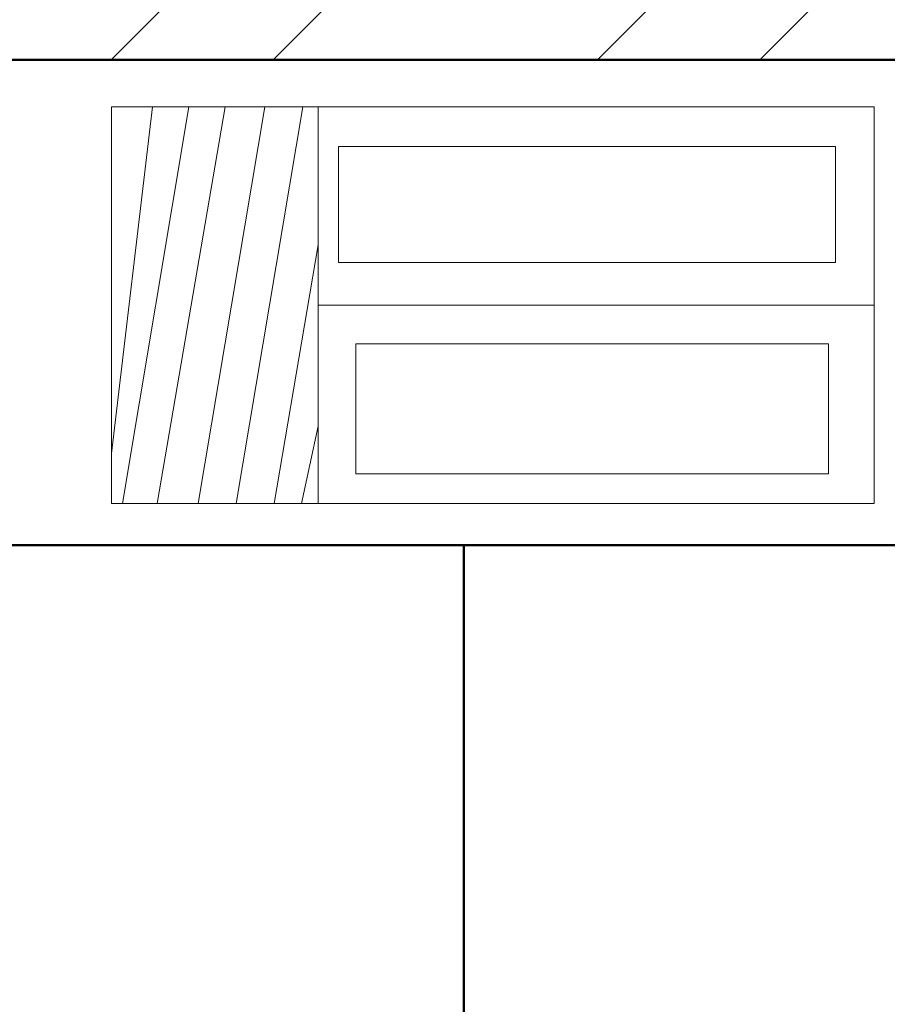
# Model space of a CAD drawing. Units: inches. Extents: x 1901 to 2863, y 888 to 2433.
# Tile 88 of 91: x 2723 to 2747, y 2052 to 2080. Entities that reach past the tile are written whole.
import ezdxf

# ---------------------------------------------------------------- set-up
doc = ezdxf.new("R2010")
doc.units = ezdxf.units.IN
for name, color, linetype, lineweight in [('A-FLOR-FIXT', 9, 'Continuous', 18), ('A-WALL', 7, 'Continuous', 50), ('A-WALL-PATT', 8, 'Continuous', 13)]:
    doc.layers.add(name, color=color, linetype=linetype, lineweight=lineweight)

msp = doc.modelspace()

# ---------------------------------------------------------------- hatches: boundary and pattern name
at = {"layer": 'A-WALL-PATT'}
h = msp.add_hatch(dxfattribs=at)
h.set_pattern_fill('ANSI32', color=256)
h.paths.add_polyline_path([(2192.501, 2274.134), (2141.264, 2274.134), (2141.264, 2269.634), (2192.501, 2269.634)])
h.paths.add_polyline_path([(2259.926, 2274.134), (2216.501, 2274.134), (2216.501, 2269.634), (2255.426, 2269.634), (2255.426, 2214.634), (2250.809, 2214.634), (2250.809, 2210.134), (2259.926, 2210.134), (2259.926, 2215.134), (2271.756, 2215.134), (2271.756, 2217.384), (2271.756, 2219.634), (2259.926, 2219.634)])
h.paths.add_polyline_path([(2171.426, 2269.634), (2166.926, 2269.634), (2166.926, 2219.634), (2121.238, 2219.634), (2121.238, 2215.134), (2166.926, 2215.134), (2166.926, 2083.134), (2161.807, 2083.134), (2161.807, 2078.634), (2171.426, 2078.634), (2176.996, 2078.634), (2176.996, 2080.884), (2176.996, 2083.134), (2171.426, 2083.134), (2171.426, 2210.134), (2230.912, 2210.134), (2230.912, 2212.384), (2230.912, 2214.634), (2171.426, 2214.634)])
h.paths.add_polyline_path([(2117.264, 2274.134), (2089.426, 2274.134), (2089.426, 2219.634), (2081.136, 2219.634), (2081.136, 2215.134), (2089.426, 2215.134), (2098.004, 2215.134), (2098.004, 2217.384), (2098.004, 2219.634), (2093.926, 2219.634), (2093.926, 2269.634), (2117.264, 2269.634), (2117.264, 2271.884)])
h.paths.add_polyline_path([(2343.426, 2219.634), (2329.295, 2219.634), (2329.295, 2215.134), (2338.926, 2215.134), (2338.926, 2184.739), (2343.426, 2184.739)])
h.paths.add_polyline_path([(2338.926, 2083.134), (2329.295, 2083.134), (2208.966, 2083.134), (2208.966, 2078.634), (2338.926, 2078.634)])
h.paths.add_polyline_path([(2343.426, 2136.739), (2338.926, 2136.739), (2338.926, 1872.634), (2343.426, 1872.634)])
h.paths.add_polyline_path([(2343.426, 1863.634), (2397.68, 1863.634), (2397.68, 1821.634), (2384.138, 1821.634), (2384.138, 1812.634), (2418.33, 1812.634), (2418.33, 1817.134), (2418.33, 1821.634), (2406.68, 1821.634), (2406.68, 1863.634), (2459.499, 1863.634), (2459.499, 1821.634), (2447.138, 1821.634), (2447.138, 1812.634), (2459.499, 1812.634), (2468.499, 1812.634), (2468.499, 1872.634), (2394.426, 1872.634), (2334.426, 1872.634), (2334.426, 1812.634), (2343.426, 1812.634), (2353.251, 1812.634), (2353.251, 1821.634), (2343.426, 1821.634)])
h.paths.add_polyline_path([(2510.014, 1872.634), (2468.499, 1872.634), (2468.499, 1868.134), (2510.014, 1868.134)])
h.paths.add_polyline_path([(2514.009, 1817.134), (2468.499, 1817.134), (2468.499, 1812.634), (2482.114, 1812.634), (2482.114, 1800.606), (2486.614, 1800.606), (2486.614, 1812.634), (2514.009, 1812.634)])
h.paths.add_polyline_path([(2299.247, 1814.884), (2299.247, 1817.134), (2295.926, 1817.134), (2295.926, 1854.169), (2293.676, 1854.169), (2291.426, 1854.169), (2291.426, 1817.134), (2266.109, 1817.134), (2266.109, 1812.634), (2299.247, 1812.634)])
h.paths.add_polyline_path([(2218.109, 1817.134), (2206.46, 1817.134), (2171.426, 1817.134), (2171.426, 1949.134), (2190.1, 1949.134), (2190.1, 1953.634), (2163.468, 1953.634), (2163.468, 1949.134), (2166.926, 1949.134), (2166.926, 1817.134), (2114.297, 1817.134), (2114.297, 1812.634), (2218.109, 1812.634)])
h.paths.add_polyline_path([(2029.426, 1970.922), (2024.926, 1970.922), (2024.926, 1912.717), (2029.426, 1912.717)])
h.paths.add_polyline_path([(2132.297, 1953.634), (2113.926, 1953.634), (2113.926, 1975.888), (2111.676, 1975.888), (2109.426, 1975.888), (2109.426, 1953.634), (2029.426, 1953.634), (2029.426, 1949.134), (2132.297, 1949.134)])
h.paths.add_polyline_path([(2029.426, 1853.606), (2029.31, 1853.606), (2029.31, 1853.606), (2029.426, 1853.606), (2029.426, 1864.717), (2024.926, 1864.717), (2024.926, 1812.634), (2066.297, 1812.634), (2066.297, 1814.884), (2066.297, 1817.134), (2029.426, 1817.134)])
h.paths.add_polyline_path([(2122.926, 2010.088), (2120.676, 2010.088), (2118.426, 2010.088), (2118.426, 2006.134), (2029.426, 2006.134), (2029.426, 2001.634), (2109.426, 2001.634), (2109.426, 1998.041), (2113.926, 1998.041), (2113.926, 2001.634), (2122.926, 2001.634)])
h.paths.add_polyline_path([(2029.426, 2031.376), (2024.926, 2031.376), (2024.926, 1994.922), (2027.176, 1994.922), (2029.426, 1994.922)])
h.paths.add_polyline_path([(2029.426, 2136.739), (2024.926, 2136.739), (2024.926, 2067.376), (2027.176, 2067.376), (2029.426, 2067.376)])
h.paths.add_polyline_path([(2125.618, 2083.134), (2029.426, 2083.134), (2029.426, 2078.634), (2118.426, 2078.634), (2118.426, 2030.715), (2122.926, 2030.715), (2122.926, 2078.634), (2125.618, 2078.634)])
h.paths.add_polyline_path([(2029.426, 2215.134), (2040.468, 2215.134), (2040.468, 2217.384), (2040.468, 2219.634), (2024.926, 2219.634), (2024.926, 2184.739), (2029.426, 2184.739), (2029.426, 2187.778)])
h.paths.add_polyline_path([(2686.426, 2274.134), (2659.284, 2274.134), (2659.284, 2269.634), (2681.926, 2269.634), (2681.926, 2219.634), (2676.816, 2219.634), (2676.816, 2215.134), (2681.926, 2215.134), (2697.011, 2215.134), (2697.011, 2217.384), (2697.011, 2219.634), (2686.426, 2219.634)])
h.paths.add_polyline_path([(2609.926, 2269.634), (2635.284, 2269.634), (2635.284, 2274.134), (2571.431, 2274.134), (2571.431, 2269.634), (2605.426, 2269.634), (2605.426, 2214.634), (2549.098, 2214.634), (2549.098, 2210.134), (2605.426, 2210.134), (2605.426, 2083.134), (2601.014, 2083.134), (2601.014, 2080.884), (2601.014, 2078.634), (2609.926, 2078.634), (2616.162, 2078.634), (2616.162, 2080.884), (2616.162, 2083.134), (2609.926, 2083.134), (2609.926, 2215.134), (2651.465, 2215.134), (2651.465, 2217.384), (2651.465, 2219.634), (2609.926, 2219.634)])
h.paths.add_polyline_path([(2521.426, 2269.634), (2547.431, 2269.634), (2547.431, 2271.884), (2547.431, 2274.134), (2516.926, 2274.134), (2516.926, 2219.634), (2506.41, 2219.634), (2506.41, 2215.134), (2516.926, 2215.134), (2516.926, 2210.134), (2525.402, 2210.134), (2525.402, 2212.384), (2525.402, 2214.634), (2521.426, 2214.634)])
h.paths.add_polyline_path([(2456.011, 2219.634), (2439.426, 2219.634), (2439.426, 2187.888), (2443.926, 2187.888), (2443.926, 2215.134), (2456.011, 2215.134)])
h.paths.add_polyline_path([(2752.926, 2219.634), (2739.485, 2219.634), (2739.485, 2215.134), (2748.426, 2215.134), (2748.426, 2187.888), (2752.926, 2187.888)])
h.paths.add_polyline_path([(2752.926, 2139.888), (2748.426, 2139.888), (2748.426, 2083.134), (2648.416, 2083.134), (2648.416, 2078.634), (2654.926, 2078.634), (2654.926, 2039.437), (2659.426, 2039.437), (2659.426, 2078.634), (2748.426, 2078.634), (2748.426, 2063.429), (2752.926, 2063.429)])
h.paths.add_polyline_path([(2752.926, 2010.634), (2659.426, 2010.634), (2659.426, 2015.652), (2654.926, 2015.652), (2654.926, 2010.634), (2605.426, 2010.634), (2605.426, 1920.967), (2609.926, 1920.967), (2609.926, 2006.134), (2748.426, 2006.134), (2748.426, 1982.466), (2752.926, 1982.466)])
h.paths.add_polyline_path([(2752.926, 2027.429), (2748.426, 2027.429), (2748.426, 2010.634), (2752.926, 2010.634)])
h.paths.add_polyline_path([(2748.426, 1886.134), (2609.926, 1886.134), (2609.926, 1889.719), (2605.426, 1889.719), (2605.426, 1861.262), (2609.926, 1861.262), (2609.926, 1881.634), (2748.426, 1881.634)])
h.paths.add_polyline_path([(2456.855, 2228.831), (2498.401, 2228.831), (2498.401, 2247.488), (2456.855, 2247.488)], flags=9)
h.paths.add_polyline_path([(2038.602, 2237.418), (2080.174, 2237.418), (2080.174, 2256.075), (2038.602, 2256.075)], flags=9)
h.paths.add_polyline_path([(2292.009, 1062.394), (2539.932, 1062.394), (2539.932, 1099.487), (2292.009, 1099.487)], flags=9)
h.paths.add_polyline_path([(2424.91, 1832.253), (2448.513, 1832.253), (2448.513, 1846.678), (2424.91, 1846.678)], flags=25)
h.paths.add_polyline_path([(2359.076, 1832.253), (2382.678, 1832.253), (2382.678, 1846.678), (2359.076, 1846.678)], flags=25)
h.paths.add_polyline_path([(2352.899, 1684.802), (2367.543, 1684.802), (2367.543, 1697.167), (2352.899, 1697.167)], flags=9)
h.paths.add_polyline_path([(2079.288, 1755.826), (2169.024, 1755.826), (2169.024, 1774.372), (2079.288, 1774.372)], flags=9)
h.paths.add_polyline_path([(2404.09, 1373.857), (2404.09, 1463.593), (2385.544, 1463.593), (2385.544, 1373.857)], flags=9)
h.paths.add_polyline_path([(2268.091, 2236.371), (2309.636, 2236.371), (2309.636, 2255.028), (2268.091, 2255.028)], flags=9)
h.paths.add_polyline_path([(2575.96, 1700.951), (2665.696, 1700.951), (2665.696, 1719.498), (2575.96, 1719.498)], flags=9)
h.paths.add_polyline_path([(2302.962, 1878.474), (2329.524, 1878.474), (2329.524, 1888.777), (2302.962, 1888.777)], flags=9)
h.paths.add_polyline_path([(2097.415, 2240.576), (2126.573, 2240.576), (2126.573, 2259.233), (2097.415, 2259.233)], flags=9)
h.paths.add_polyline_path([(2208.725, 2246.124), (2237.882, 2246.124), (2237.882, 2264.781), (2208.725, 2264.781)], flags=9)
h.paths.add_polyline_path([(2038.147, 1925.958), (2076.987, 1925.958), (2076.987, 1944.615), (2038.147, 1944.615)], flags=9)
h.paths.add_polyline_path([(2239.144, 1926.672), (2288.465, 1926.672), (2288.465, 1945.329), (2239.144, 1945.329)], flags=9)
h.paths.add_polyline_path([(2175.429, 2007.33), (2212.356, 2007.33), (2212.356, 2025.987), (2175.429, 2025.987)], flags=9)
h.paths.add_polyline_path([(2225.034, 2091.794), (2263.875, 2091.794), (2263.875, 2110.451), (2225.034, 2110.451)], flags=9)
h.paths.add_polyline_path([(2035.398, 2098.478), (2074.238, 2098.478), (2074.238, 2117.135), (2035.398, 2117.135)], flags=9)
h.paths.add_polyline_path([(2050.102, 2029.209), (2083.26, 2029.209), (2083.26, 2047.866), (2050.102, 2047.866)], flags=9)
h.paths.add_polyline_path([(2069.677, 1956.719), (2098.835, 1956.719), (2098.835, 1975.376), (2069.677, 1975.376)], flags=25)
h.paths.add_polyline_path([(2328.62, 1753.336), (2361.663, 1753.336), (2361.663, 1771.993), (2328.62, 1771.993)], flags=9)
h.paths.add_polyline_path([(2395.162, 2060.888), (2395.162, 2140.654), (2378.676, 2140.654), (2378.676, 2060.888)], flags=9)
h.paths.add_polyline_path([(2463.728, 2059.02), (2492.886, 2059.02), (2492.886, 2077.677), (2463.728, 2077.677)], flags=9)
h.paths.add_polyline_path([(2458.027, 2181.536), (2496.868, 2181.536), (2496.868, 2200.194), (2458.027, 2200.194)], flags=9)
h.paths.add_polyline_path([(2527.577, 2243.074), (2556.735, 2243.074), (2556.735, 2261.731), (2527.577, 2261.731)], flags=9)
h.paths.add_polyline_path([(2694.461, 2232.767), (2736.033, 2232.767), (2736.033, 2251.425), (2694.461, 2251.425)], flags=9)
h.paths.add_polyline_path([(2637.821, 2249.225), (2666.979, 2249.225), (2666.979, 2267.882), (2637.821, 2267.882)], flags=9)
h.paths.add_polyline_path([(2623.687, 2183.541), (2662.528, 2183.541), (2662.528, 2202.199), (2623.687, 2202.199)], flags=9)
h.paths.add_polyline_path([(2691.965, 2021.5), (2725.124, 2021.5), (2725.124, 2040.157), (2691.965, 2040.157)], flags=9)
h.paths.add_polyline_path([(2621.043, 1975.912), (2662.335, 1975.912), (2662.335, 1994.569), (2621.043, 1994.569)], flags=25)
h.paths.add_polyline_path([(2479.032, 1927.62), (2519.844, 1927.62), (2519.844, 1946.277), (2479.032, 1946.277)], flags=9)
h.paths.add_polyline_path([(2670.941, 1849.076), (2716.005, 1849.076), (2716.005, 1867.734), (2670.941, 1867.734)], flags=9)
h.paths.add_polyline_path([(2523.613, 1782.956), (2550.175, 1782.956), (2550.175, 1793.26), (2523.613, 1793.26)], flags=9)
h.paths.add_polyline_path([(2450.841, 1207.331), (2492.386, 1207.331), (2492.386, 1225.989), (2450.841, 1225.989)], flags=9)
h.paths.add_polyline_path([(2527.751, 1203.841), (2556.908, 1203.841), (2556.908, 1222.499), (2527.751, 1222.499)], flags=9)
h.paths.add_polyline_path([(2639.111, 1207.2), (2668.268, 1207.2), (2668.268, 1225.857), (2639.111, 1225.857)], flags=9)
h.paths.add_polyline_path([(2692.594, 1218.965), (2734.167, 1218.965), (2734.167, 1237.623), (2692.594, 1237.623)], flags=9)
h.paths.add_polyline_path([(2669.266, 1366.329), (2708.106, 1366.329), (2708.106, 1384.987), (2669.266, 1384.987)], flags=9)
h.paths.add_polyline_path([(2463.313, 1358.031), (2502.153, 1358.031), (2502.153, 1376.688), (2463.313, 1376.688)], flags=9)
h.paths.add_polyline_path([(2494.725, 1449.963), (2531.652, 1449.963), (2531.652, 1468.62), (2494.725, 1468.62)], flags=9)
h.paths.add_polyline_path([(2675.565, 1422.157), (2708.724, 1422.157), (2708.724, 1440.815), (2675.565, 1440.815)], flags=9)
h.paths.add_polyline_path([(2685.634, 1493.891), (2714.792, 1493.891), (2714.792, 1512.548), (2685.634, 1512.548)], flags=9)
h.paths.add_polyline_path([(2686.805, 1529.913), (2725.645, 1529.913), (2725.645, 1548.57), (2686.805, 1548.57)], flags=9)
h.paths.add_polyline_path([(2503.651, 1537.991), (2552.972, 1537.991), (2552.972, 1556.648), (2503.651, 1556.648)], flags=9)
h.paths.add_polyline_path([(2291.713, 1643.504), (2318.275, 1643.504), (2318.275, 1653.807), (2291.713, 1653.807)], flags=9)
h.paths.add_polyline_path([(2450.626, 1610.52), (2477.189, 1610.52), (2477.189, 1620.824), (2450.626, 1620.824)], flags=9)
h.paths.add_polyline_path([(2359.985, 1551.814), (2422.253, 1551.814), (2422.253, 1562.117), (2359.985, 1562.117)], flags=9)
h.paths.add_polyline_path([(2280.106, 1249.006), (2321.651, 1249.006), (2321.651, 1267.663), (2280.106, 1267.663)], flags=9)
h.paths.add_polyline_path([(2164.057, 1274.232), (2193.215, 1274.232), (2193.215, 1292.889), (2164.057, 1292.889)], flags=9)
h.paths.add_polyline_path([(2118.21, 1277.694), (2151.252, 1277.694), (2151.252, 1296.351), (2118.21, 1296.351)], flags=9)
h.paths.add_polyline_path([(2031.946, 1268.529), (2073.519, 1268.529), (2073.519, 1287.187), (2031.946, 1287.187)], flags=9)
h.paths.add_polyline_path([(2050.199, 1409.079), (2089.04, 1409.079), (2089.04, 1427.736), (2050.199, 1427.736)], flags=9)
h.paths.add_polyline_path([(2243.743, 1421.032), (2282.584, 1421.032), (2282.584, 1439.689), (2243.743, 1439.689)], flags=9)
h.paths.add_polyline_path([(2190.746, 1509.769), (2231.558, 1509.769), (2231.558, 1528.426), (2190.746, 1528.426)], flags=9)
h.paths.add_polyline_path([(2058.392, 1475.415), (2091.55, 1475.415), (2091.55, 1494.073), (2058.392, 1494.073)], flags=9)
h.paths.add_polyline_path([(2062.447, 1553.09), (2091.605, 1553.09), (2091.605, 1571.747), (2062.447, 1571.747)], flags=9)
h.paths.add_polyline_path([(2219.524, 1590.365), (2266.147, 1590.365), (2266.147, 1609.022), (2219.524, 1609.022)], flags=9)
h.paths.add_polyline_path([(2041.072, 1584.188), (2079.912, 1584.188), (2079.912, 1602.845), (2041.072, 1602.845)], flags=9)

# ---------------------------------------------------------------- linework, layer by layer
at = {"layer": 'A-FLOR-FIXT'}
for p, q in [((2726.359, 2077.331), (2725.227, 2067.734)), ((2727.365, 2077.331), (2725.532, 2066.351)), ((2728.371, 2077.331), (2726.359, 2077.331)), ((2728.371, 2077.331), (2726.492, 2066.351)), ((2729.469, 2077.331), (2727.63, 2066.351)), ((2730.525, 2077.331), (2728.682, 2066.351)), ((2730.949, 2077.331), (2730.949, 2066.351)), ((2730.949, 2077.331), (2730.949, 2077.331)), ((2730.949, 2073.512), (2729.726, 2066.351)), ((2730.949, 2071.841), (2746.336, 2071.841)), ((2730.949, 2068.487), (2730.488, 2066.351)), ((2730.174, 2066.351), (2728.371, 2066.351))]:
    msp.add_line(p, q, dxfattribs=at)
for points in [[(2725.227, 2077.331), (2746.336, 2077.331), (2746.336, 2066.351), (2725.227, 2066.351)], [(2731.513, 2076.235), (2745.272, 2076.235), (2745.272, 2073.017), (2731.513, 2073.017)], [(2731.994, 2070.773), (2745.072, 2070.773), (2745.072, 2067.168), (2731.994, 2067.168)]]:
    msp.add_lwpolyline(points, close=True, dxfattribs=at)
at = {"layer": 'A-WALL'}
for p, q in [((2659.426, 2078.634), (2748.426, 2078.634)), ((2659.426, 2065.199), (2734.984, 2065.199)), ((2734.984, 2065.199), (2734.984, 2010.634)), ((2734.984, 2065.199), (2748.426, 2065.199))]:
    msp.add_line(p, q, dxfattribs=at)

doc.saveas('drawing.dxf')
